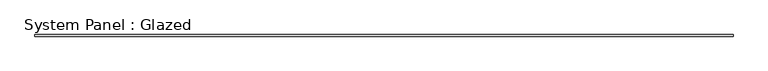
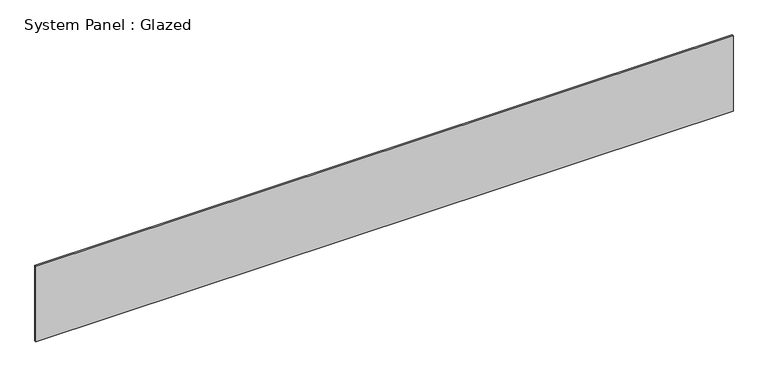
"""IFC4 building model written with IfcOpenShell, lengths in millimetres: plate geometry, System Panel : Glazed."""

from ifc_helpers import new_model, si_unit, origin, origin_with_axes, place, context, project, spatial, polyline, outline, extrude, source, transform, mapped, element, save


def system_panel_glazed_0f212477(model_context):
    return source(origin(), model_context, "Body", "SweptSolid", [
        extrude(outline(polyline([(5334.0, 19.05), (-5334.0, 19.05), (-5334.0, 44.45), (5334.0, 44.45), (5334.0, 19.05)])), origin_with_axes(), (0.0, 0.0, 1.0), 1219.2),
    ])


if __name__ == "__main__":
    model = new_model("IFC4")
    model_context = context("Model", 3, world=origin())
    ifc_project = project(units=[si_unit("LENGTHUNIT", "METRE", prefix="MILLI")], contexts=[model_context])
    site = spatial("IfcSite", under=ifc_project)
    building = spatial("IfcBuilding", under=site)
    placement = place(None, origin())
    system_panel_glazed_shape = system_panel_glazed_0f212477(model_context)
    element("IfcPlate", 1, ObjectType="System Panel : Glazed", at=placement, inside=building, context=model_context, shape_type="MappedRepresentation", body=[
        mapped(system_panel_glazed_shape, transform((0.0, 0.0, 0.0), x_axis=(1.0, 0.0, 0.0), y_axis=(0.0, 1.0, 0.0), z_axis=(0.0, 0.0, 1.0))),
    ])
    save(model, "model.ifc")

# Revit data of these elements
# Type "System Panel : Glazed"
#   Construction Type Id = "GSP4R"
#   Analytic Construction = "1/8 in Pilkington single glazing"
#   Visual Light Transmittance = 0.9
#   Solar Heat Gain Coefficient = 0.86
#   Heat Transfer Coefficient (U) = 1.18115 BTU/(h·ft²·°F)
# Element 1 (IfcPlate, "System Panel : Glazed")
#   Materials on its faces: "Glass"
# Materials
#   "Glass": class "Glass", colour RGB 0 128 192, transparency 0.75, Description = "Soda Lime Glass", Cost = 0
